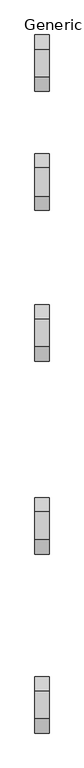
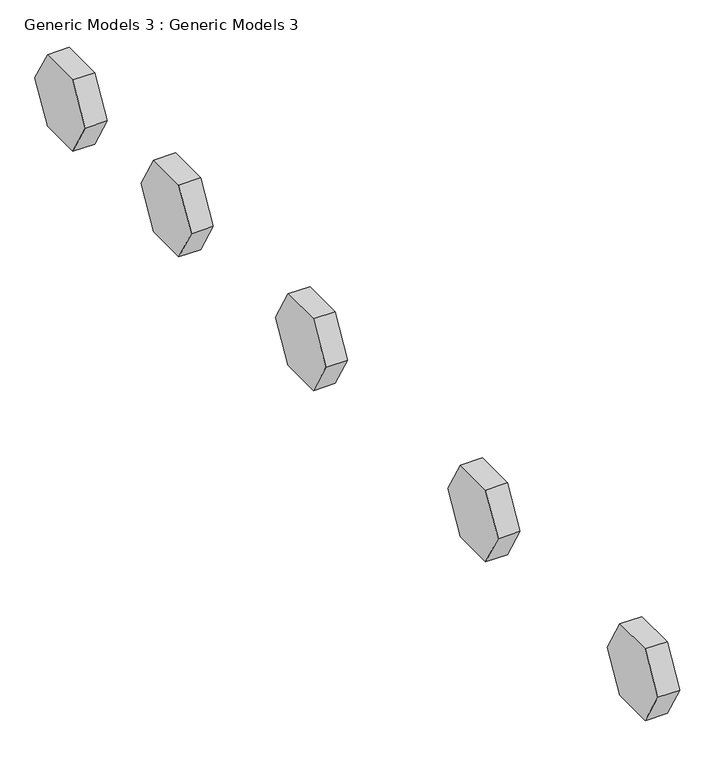
"""IFC4 building model written with IfcOpenShell, lengths in millimetres: proxy geometry, Generic Models 3 : Generic Models 3."""

from ifc_helpers import new_model, si_unit, frame, origin, place, context, project, spatial, polyline, outline, extrude, source, transform, mapped, element, save


def generic_models_3_generic_models_3_c1cfd057(model_context):
    return source(origin(), model_context, "Body", "SweptSolid", [
        extrude(outline(polyline([(-6745.6556704, 1290.0052861), (-6440.8556704, 762.0762), (-6745.6556704, 234.1471139), (-7355.2556704, 234.1471139), (-7660.0556704, 762.0762), (-7355.2556704, 1290.0052861), (-6745.6556704, 1290.0052861)])), frame((4175.6127609, 0.0, 0.0), z_axis=(1.0, 0.0, 0.0), x_axis=(0.0, 1.0, 0.0)), (0.0, 0.0, 1.0), 304.8),
        extrude(outline(polyline([(-2884.8556704, 1290.0052861), (-2580.0556704, 762.0762), (-2884.8556704, 234.1471139), (-3494.4556704, 234.1471139), (-3799.2556704, 762.0762), (-3494.4556704, 1290.0052861), (-2884.8556704, 1290.0052861)])), frame((4175.6127609, 0.0, 0.0), z_axis=(1.0, 0.0, 0.0), x_axis=(0.0, 1.0, 0.0)), (0.0, 0.0, 1.0), 304.8),
        extrude(outline(polyline([(1280.7443296, 1290.0052861), (1585.5443296, 762.0762), (1280.7443296, 234.1471139), (671.1443296, 234.1471139), (366.3443296, 762.0762), (671.1443296, 1290.0052861), (1280.7443296, 1290.0052861)])), frame((4175.6127609, 0.0, 0.0), z_axis=(1.0, 0.0, 0.0), x_axis=(0.0, 1.0, 0.0)), (0.0, 0.0, 1.0), 304.8),
        extrude(outline(polyline([(4531.9443296, 1290.0052861), (4836.7443296, 762.0762), (4531.9443296, 234.1471139), (3922.3443296, 234.1471139), (3617.5443296, 762.0762), (3922.3443296, 1290.0052861), (4531.9443296, 1290.0052861)])), frame((4175.6127609, 0.0, 0.0), z_axis=(1.0, 0.0, 0.0), x_axis=(0.0, 1.0, 0.0)), (0.0, 0.0, 1.0), 304.8),
        extrude(outline(polyline([(7097.3443296, 1290.0052861), (7402.1443296, 762.0762), (7097.3443296, 234.1471139), (6487.7443296, 234.1471139), (6182.9443296, 762.0762), (6487.7443296, 1290.0052861), (7097.3443296, 1290.0052861)])), frame((4175.6127609, 0.0, 0.0), z_axis=(1.0, 0.0, 0.0), x_axis=(0.0, 1.0, 0.0)), (0.0, 0.0, 1.0), 304.8),
    ])


if __name__ == "__main__":
    model = new_model("IFC4")
    model_context = context("Model", 3, world=origin())
    ifc_project = project(units=[si_unit("LENGTHUNIT", "METRE", prefix="MILLI")], contexts=[model_context])
    site = spatial("IfcSite", under=ifc_project)
    building = spatial("IfcBuilding", under=site)
    placement = place(None, origin())
    generic_models_3_generic_models_3_shape = generic_models_3_generic_models_3_c1cfd057(model_context)
    element("IfcBuildingElementProxy", 1, Name="Generic Models 3 : Generic Models 3", ObjectType="Generic Models 3 : Generic Models 3", at=placement, inside=building, context=model_context, shape_type="MappedRepresentation", body=[
        mapped(generic_models_3_generic_models_3_shape, transform((0.0, 0.0, 0.0), x_axis=(1.0, 0.0, 0.0), y_axis=(0.0, 1.0, 0.0), z_axis=(0.0, 0.0, 1.0))),
    ])
    save(model, "model.ifc")

# Revit data of these elements
# Element 1 (IfcBuildingElementProxy, "Generic Models 3 : Generic Models 3")
#   Materials on its faces: "Clad - White", "Concrete Masonry Units"
# Materials
#   "Clad - White": class "Wood", colour RGB 242 242 238, transparency 0, Cost = 0
#   "Concrete Masonry Units": class "Masonry", colour RGB 227 227 227, transparency 0, Description = "Concrete masonry units", Cost = 0
